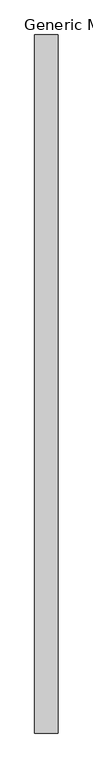
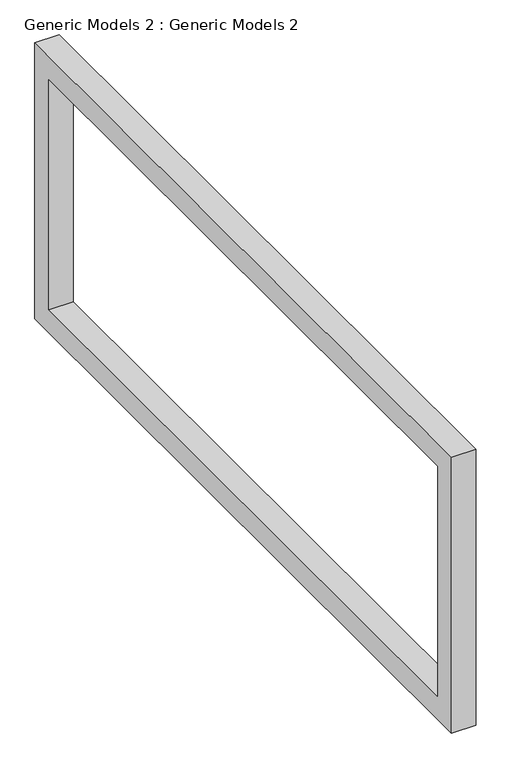
"""IFC4 building model written with IfcOpenShell, lengths in millimetres: proxy geometry, Generic Models 2 : Generic Models 2."""

from ifc_helpers import new_model, si_unit, frame, origin, place, context, project, spatial, polyline, outline, extrude, source, transform, mapped, element, save


def generic_models_2_generic_models_2_29e6902f(model_context):
    return source(origin(), model_context, "Body", "SweptSolid", [
        extrude(outline(polyline([(4131.1500875, 6400.8), (4131.1500875, 2743.2), (-4923.9499125, 2743.2), (-4923.9499125, 6400.8), (4131.1500875, 6400.8)]), holes=[polyline([(3826.3500875, 6096.0), (-4619.1499125, 6096.0), (-4619.1499125, 3048.0), (3826.3500875, 3048.0), (3826.3500875, 6096.0)])]), frame((-2255.7656154, 0.0, 0.0), z_axis=(1.0, 0.0, 0.0), x_axis=(0.0, 1.0, 0.0)), (0.0, 0.0, 1.0), 304.8),
    ])


if __name__ == "__main__":
    model = new_model("IFC4")
    model_context = context("Model", 3, world=origin())
    ifc_project = project(units=[si_unit("LENGTHUNIT", "METRE", prefix="MILLI")], contexts=[model_context])
    site = spatial("IfcSite", under=ifc_project)
    building = spatial("IfcBuilding", under=site)
    placement = place(None, origin())
    generic_models_2_generic_models_2_shape = generic_models_2_generic_models_2_29e6902f(model_context)
    element("IfcBuildingElementProxy", 1, Name="Generic Models 2 : Generic Models 2", ObjectType="Generic Models 2 : Generic Models 2", at=placement, inside=building, context=model_context, shape_type="MappedRepresentation", body=[
        mapped(generic_models_2_generic_models_2_shape, transform((0.0, 0.0, 0.0), x_axis=(1.0, 0.0, 0.0), y_axis=(0.0, 1.0, 0.0), z_axis=(0.0, 0.0, 1.0))),
    ])
    save(model, "model.ifc")

# Revit data of these elements
# Element 1 (IfcBuildingElementProxy, "Generic Models 2 : Generic Models 2")
#   Materials on its faces: "LIGHT BEIGE"
# Materials
#   "LIGHT BEIGE": class "Generic", colour RGB 120 120 120, transparency 0, Cost = 0
